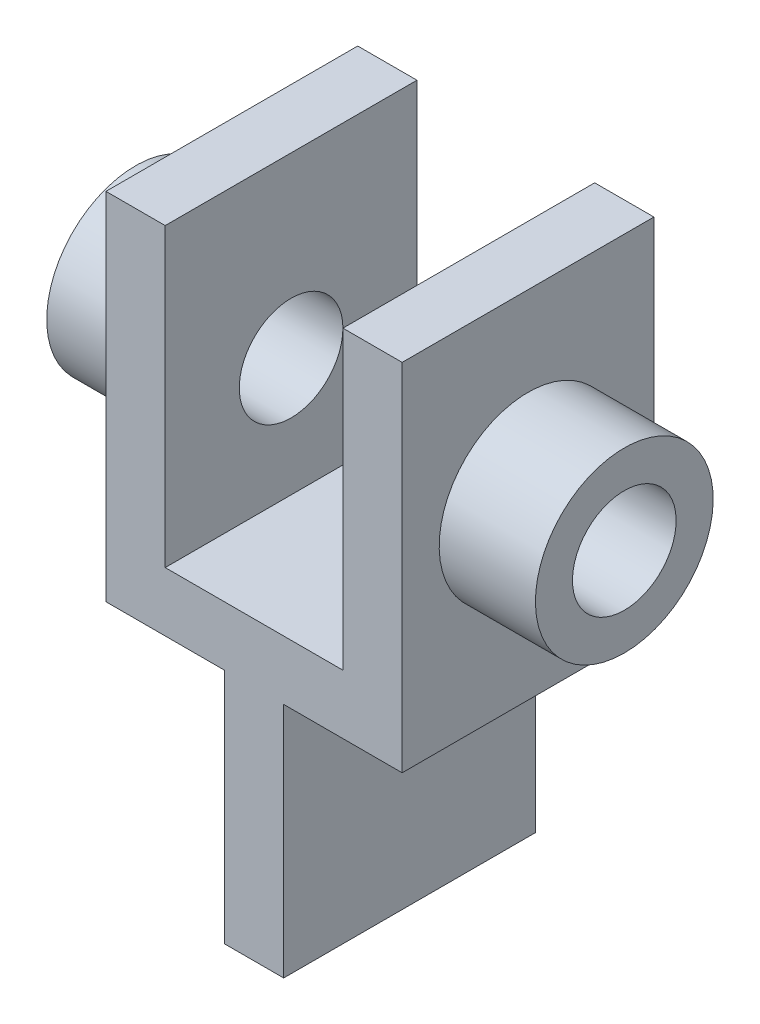
ISO-10303-21;
HEADER;
FILE_DESCRIPTION(('STEP AP214'),'2;1');
FILE_NAME('part.step','',(''),(''),'','','');
FILE_SCHEMA(('AUTOMOTIVE_DESIGN { 1 0 10303 214 1 1 1 1 }'));
ENDSEC;
DATA;
#1=APPLICATION_CONTEXT('core data for automotive mechanical design processes');
#2=APPLICATION_PROTOCOL_DEFINITION('international standard','automotive_design',2000,#1);
#3=PRODUCT_CONTEXT('',#1,'mechanical');
#4=PRODUCT('Part','Part','',(#3));
#5=PRODUCT_RELATED_PRODUCT_CATEGORY('part','',(#4));
#6=PRODUCT_DEFINITION_FORMATION('','',#4);
#7=PRODUCT_DEFINITION_CONTEXT('part definition',#1,'design');
#8=PRODUCT_DEFINITION('design','',#6,#7);
#9=PRODUCT_DEFINITION_SHAPE('','',#8);
#10=(LENGTH_UNIT() NAMED_UNIT(*) SI_UNIT(.MILLI.,.METRE.));
#11=(NAMED_UNIT(*) PLANE_ANGLE_UNIT() SI_UNIT($,.RADIAN.));
#12=(NAMED_UNIT(*) SI_UNIT($,.STERADIAN.) SOLID_ANGLE_UNIT());
#13=UNCERTAINTY_MEASURE_WITH_UNIT(LENGTH_MEASURE(1.E-05),#10,'distance_accuracy_value','');
#14=(GEOMETRIC_REPRESENTATION_CONTEXT(3) GLOBAL_UNCERTAINTY_ASSIGNED_CONTEXT((#13)) GLOBAL_UNIT_ASSIGNED_CONTEXT((#10,
#11,#12)) REPRESENTATION_CONTEXT('',''));
#15=CARTESIAN_POINT('',(0.,0.,0.));
#16=DIRECTION('',(0.,0.,1.));
#17=DIRECTION('',(1.,0.,0.));
#18=AXIS2_PLACEMENT_3D('',#15,#16,#17);
#19=CARTESIAN_POINT('',(-2.8719126938541,0.,-34.));
#20=DIRECTION('',(0.,-1.,0.));
#21=DIRECTION('',(0.,0.,-1.));
#22=AXIS2_PLACEMENT_3D('',#19,#20,#21);
#23=PLANE('',#22);
#24=DIRECTION('',(1.,0.,0.));
#25=VECTOR('',#24,1.);
#26=CARTESIAN_POINT('',(-2.8719126938541,0.,0.));
#27=LINE('',#26,#25);
#28=CARTESIAN_POINT('',(-2.8719126938541,0.,0.));
#29=VERTEX_POINT('',#28);
#30=CARTESIAN_POINT('',(5.1280873061459,0.,0.));
#31=VERTEX_POINT('',#30);
#32=EDGE_CURVE('E165',#29,#31,#27,.T.);
#33=ORIENTED_EDGE('',*,*,#32,.F.);
#34=DIRECTION('',(0.,0.,1.));
#35=VECTOR('',#34,1.);
#36=CARTESIAN_POINT('',(-2.8719126938541,0.,-34.));
#37=LINE('',#36,#35);
#38=CARTESIAN_POINT('',(-2.8719126938541,0.,-34.));
#39=VERTEX_POINT('',#38);
#40=EDGE_CURVE('E11',#39,#29,#37,.T.);
#41=ORIENTED_EDGE('',*,*,#40,.F.);
#42=DIRECTION('',(1.,0.,0.));
#43=VECTOR('',#42,1.);
#44=CARTESIAN_POINT('',(-2.8719126938541,0.,-34.));
#45=LINE('',#44,#43);
#46=CARTESIAN_POINT('',(5.1280873061459,0.,-34.));
#47=VERTEX_POINT('',#46);
#48=EDGE_CURVE('E192',#39,#47,#45,.T.);
#49=ORIENTED_EDGE('',*,*,#48,.T.);
#50=DIRECTION('',(0.,0.,1.));
#51=VECTOR('',#50,1.);
#52=CARTESIAN_POINT('',(5.1280873061459,0.,-34.));
#53=LINE('',#52,#51);
#54=EDGE_CURVE('E42',#47,#31,#53,.T.);
#55=ORIENTED_EDGE('',*,*,#54,.T.);
#56=EDGE_LOOP('',(#33,#41,#49,#55));
#57=FACE_BOUND('',#56,.T.);
#58=ADVANCED_FACE('F41',(#57),#23,.T.);
#59=CARTESIAN_POINT('',(-2.8719126938541,0.,-34.));
#60=DIRECTION('',(-1.,0.,0.));
#61=DIRECTION('',(0.,0.,1.));
#62=AXIS2_PLACEMENT_3D('',#59,#60,#61);
#63=PLANE('',#62);
#64=DIRECTION('',(0.,-1.,0.));
#65=VECTOR('',#64,1.);
#66=CARTESIAN_POINT('',(-2.8719126938541,0.,0.));
#67=LINE('',#66,#65);
#68=CARTESIAN_POINT('',(-2.8719126938541,32.,0.));
#69=VERTEX_POINT('',#68);
#70=EDGE_CURVE('E191',#69,#29,#67,.T.);
#71=ORIENTED_EDGE('',*,*,#70,.F.);
#72=DIRECTION('',(0.,0.,1.));
#73=VECTOR('',#72,1.);
#74=CARTESIAN_POINT('',(-2.8719126938541,32.,-34.));
#75=LINE('',#74,#73);
#76=CARTESIAN_POINT('',(-2.8719126938541,32.,-34.));
#77=VERTEX_POINT('',#76);
#78=EDGE_CURVE('E49',#77,#69,#75,.T.);
#79=ORIENTED_EDGE('',*,*,#78,.F.);
#80=DIRECTION('',(0.,-1.,0.));
#81=VECTOR('',#80,1.);
#82=CARTESIAN_POINT('',(-2.8719126938541,0.,-34.));
#83=LINE('',#82,#81);
#84=EDGE_CURVE('E155',#77,#39,#83,.T.);
#85=ORIENTED_EDGE('',*,*,#84,.T.);
#86=ORIENTED_EDGE('',*,*,#40,.T.);
#87=EDGE_LOOP('',(#71,#79,#85,#86));
#88=FACE_BOUND('',#87,.T.);
#89=ADVANCED_FACE('F214',(#88),#63,.T.);
#90=CARTESIAN_POINT('',(-2.8719126938541,32.,-34.));
#91=DIRECTION('',(0.,-1.,0.));
#92=DIRECTION('',(1.,0.,0.));
#93=AXIS2_PLACEMENT_3D('',#90,#91,#92);
#94=PLANE('',#93);
#95=DIRECTION('',(1.,0.,0.));
#96=VECTOR('',#95,1.);
#97=CARTESIAN_POINT('',(-2.8719126938541,32.,0.));
#98=LINE('',#97,#96);
#99=CARTESIAN_POINT('',(-18.8719126938541,32.,0.));
#100=VERTEX_POINT('',#99);
#101=EDGE_CURVE('E139',#100,#69,#98,.T.);
#102=ORIENTED_EDGE('',*,*,#101,.F.);
#103=DIRECTION('',(0.,0.,1.));
#104=VECTOR('',#103,1.);
#105=CARTESIAN_POINT('',(-18.8719126938541,32.,-34.));
#106=LINE('',#105,#104);
#107=CARTESIAN_POINT('',(-18.8719126938541,32.,-34.));
#108=VERTEX_POINT('',#107);
#109=EDGE_CURVE('E134',#108,#100,#106,.T.);
#110=ORIENTED_EDGE('',*,*,#109,.F.);
#111=DIRECTION('',(1.,0.,0.));
#112=VECTOR('',#111,1.);
#113=CARTESIAN_POINT('',(-2.8719126938541,32.,-34.));
#114=LINE('',#113,#112);
#115=EDGE_CURVE('E140',#108,#77,#114,.T.);
#116=ORIENTED_EDGE('',*,*,#115,.T.);
#117=ORIENTED_EDGE('',*,*,#78,.T.);
#118=EDGE_LOOP('',(#102,#110,#116,#117));
#119=FACE_BOUND('',#118,.T.);
#120=ADVANCED_FACE('F138',(#119),#94,.T.);
#121=CARTESIAN_POINT('',(-18.8719126938541,32.,-34.));
#122=DIRECTION('',(-1.,0.,0.));
#123=DIRECTION('',(0.,0.,1.));
#124=AXIS2_PLACEMENT_3D('',#121,#122,#123);
#125=PLANE('',#124);
#126=CARTESIAN_POINT('',(-18.8719126938541,56.,-17.));
#127=DIRECTION('',(-1.,0.,0.));
#128=DIRECTION('',(0.,0.,1.));
#129=AXIS2_PLACEMENT_3D('',#126,#127,#128);
#130=CIRCLE('',#129,12.);
#131=CARTESIAN_POINT('',(-18.8719126938541,56.,-29.));
#132=VERTEX_POINT('',#131);
#133=EDGE_CURVE('E296',#132,#132,#130,.T.);
#134=ORIENTED_EDGE('',*,*,#133,.F.);
#135=EDGE_LOOP('',(#134));
#136=FACE_BOUND('',#135,.T.);
#137=DIRECTION('',(0.,-1.,0.));
#138=VECTOR('',#137,1.);
#139=CARTESIAN_POINT('',(-18.8719126938541,32.,0.));
#140=LINE('',#139,#138);
#141=CARTESIAN_POINT('',(-18.8719126938541,80.,0.));
#142=VERTEX_POINT('',#141);
#143=EDGE_CURVE('E187',#142,#100,#140,.T.);
#144=ORIENTED_EDGE('',*,*,#143,.F.);
#145=DIRECTION('',(0.,0.,1.));
#146=VECTOR('',#145,1.);
#147=CARTESIAN_POINT('',(-18.8719126938541,80.,-34.));
#148=LINE('',#147,#146);
#149=CARTESIAN_POINT('',(-18.8719126938541,80.,-34.));
#150=VERTEX_POINT('',#149);
#151=EDGE_CURVE('E145',#150,#142,#148,.T.);
#152=ORIENTED_EDGE('',*,*,#151,.F.);
#153=DIRECTION('',(0.,-1.,0.));
#154=VECTOR('',#153,1.);
#155=CARTESIAN_POINT('',(-18.8719126938541,32.,-34.));
#156=LINE('',#155,#154);
#157=EDGE_CURVE('E147',#150,#108,#156,.T.);
#158=ORIENTED_EDGE('',*,*,#157,.T.);
#159=ORIENTED_EDGE('',*,*,#109,.T.);
#160=EDGE_LOOP('',(#144,#152,#158,#159));
#161=FACE_BOUND('',#160,.T.);
#162=ADVANCED_FACE('F152',(#136,#161),#125,.T.);
#163=CARTESIAN_POINT('',(-18.8719126938541,80.,-34.));
#164=DIRECTION('',(0.,1.,0.));
#165=DIRECTION('',(0.,0.,1.));
#166=AXIS2_PLACEMENT_3D('',#163,#164,#165);
#167=PLANE('',#166);
#168=DIRECTION('',(-1.,0.,0.));
#169=VECTOR('',#168,1.);
#170=CARTESIAN_POINT('',(-18.8719126938541,80.,0.));
#171=LINE('',#170,#169);
#172=CARTESIAN_POINT('',(-10.8719126938541,80.,0.));
#173=VERTEX_POINT('',#172);
#174=EDGE_CURVE('E190',#173,#142,#171,.T.);
#175=ORIENTED_EDGE('',*,*,#174,.F.);
#176=DIRECTION('',(0.,0.,1.));
#177=VECTOR('',#176,1.);
#178=CARTESIAN_POINT('',(-10.8719126938541,80.,-34.));
#179=LINE('',#178,#177);
#180=CARTESIAN_POINT('',(-10.8719126938541,80.,-34.));
#181=VERTEX_POINT('',#180);
#182=EDGE_CURVE('E200',#181,#173,#179,.T.);
#183=ORIENTED_EDGE('',*,*,#182,.F.);
#184=DIRECTION('',(-1.,0.,0.));
#185=VECTOR('',#184,1.);
#186=CARTESIAN_POINT('',(-18.8719126938541,80.,-34.));
#187=LINE('',#186,#185);
#188=EDGE_CURVE('E154',#181,#150,#187,.T.);
#189=ORIENTED_EDGE('',*,*,#188,.T.);
#190=ORIENTED_EDGE('',*,*,#151,.T.);
#191=EDGE_LOOP('',(#175,#183,#189,#190));
#192=FACE_BOUND('',#191,.T.);
#193=ADVANCED_FACE('F226',(#192),#167,.T.);
#194=CARTESIAN_POINT('',(-10.8719126938541,80.,-34.));
#195=DIRECTION('',(1.,0.,0.));
#196=DIRECTION('',(0.,1.,0.));
#197=AXIS2_PLACEMENT_3D('',#194,#195,#196);
#198=PLANE('',#197);
#199=CARTESIAN_POINT('',(-10.8719126938541,56.,-17.));
#200=DIRECTION('',(1.,0.,0.));
#201=DIRECTION('',(0.,1.,0.));
#202=AXIS2_PLACEMENT_3D('',#199,#200,#201);
#203=CIRCLE('',#202,7.);
#204=CARTESIAN_POINT('',(-10.8719126938541,56.,-24.));
#205=VERTEX_POINT('',#204);
#206=EDGE_CURVE('E293',#205,#205,#203,.T.);
#207=ORIENTED_EDGE('',*,*,#206,.F.);
#208=EDGE_LOOP('',(#207));
#209=FACE_BOUND('',#208,.T.);
#210=DIRECTION('',(0.,1.,0.));
#211=VECTOR('',#210,1.);
#212=CARTESIAN_POINT('',(-10.8719126938541,80.,0.));
#213=LINE('',#212,#211);
#214=CARTESIAN_POINT('',(-10.8719126938541,40.,0.));
#215=VERTEX_POINT('',#214);
#216=EDGE_CURVE('E184',#215,#173,#213,.T.);
#217=ORIENTED_EDGE('',*,*,#216,.F.);
#218=DIRECTION('',(0.,0.,1.));
#219=VECTOR('',#218,1.);
#220=CARTESIAN_POINT('',(-10.8719126938541,40.,-34.));
#221=LINE('',#220,#219);
#222=CARTESIAN_POINT('',(-10.8719126938541,40.,-34.));
#223=VERTEX_POINT('',#222);
#224=EDGE_CURVE('E203',#223,#215,#221,.T.);
#225=ORIENTED_EDGE('',*,*,#224,.F.);
#226=DIRECTION('',(0.,1.,0.));
#227=VECTOR('',#226,1.);
#228=CARTESIAN_POINT('',(-10.8719126938541,80.,-34.));
#229=LINE('',#228,#227);
#230=EDGE_CURVE('E160',#223,#181,#229,.T.);
#231=ORIENTED_EDGE('',*,*,#230,.T.);
#232=ORIENTED_EDGE('',*,*,#182,.T.);
#233=EDGE_LOOP('',(#217,#225,#231,#232));
#234=FACE_BOUND('',#233,.T.);
#235=ADVANCED_FACE('F235',(#209,#234),#198,.T.);
#236=CARTESIAN_POINT('',(-10.8719126938541,40.,-34.));
#237=DIRECTION('',(0.,1.,0.));
#238=DIRECTION('',(-1.,0.,0.));
#239=AXIS2_PLACEMENT_3D('',#236,#237,#238);
#240=PLANE('',#239);
#241=DIRECTION('',(-1.,0.,0.));
#242=VECTOR('',#241,1.);
#243=CARTESIAN_POINT('',(-10.8719126938541,40.,0.));
#244=LINE('',#243,#242);
#245=CARTESIAN_POINT('',(13.1280873061459,40.,0.));
#246=VERTEX_POINT('',#245);
#247=EDGE_CURVE('E182',#246,#215,#244,.T.);
#248=ORIENTED_EDGE('',*,*,#247,.F.);
#249=DIRECTION('',(0.,0.,1.));
#250=VECTOR('',#249,1.);
#251=CARTESIAN_POINT('',(13.1280873061459,40.,-34.));
#252=LINE('',#251,#250);
#253=CARTESIAN_POINT('',(13.1280873061459,40.,-34.));
#254=VERTEX_POINT('',#253);
#255=EDGE_CURVE('E201',#254,#246,#252,.T.);
#256=ORIENTED_EDGE('',*,*,#255,.F.);
#257=DIRECTION('',(-1.,0.,0.));
#258=VECTOR('',#257,1.);
#259=CARTESIAN_POINT('',(-10.8719126938541,40.,-34.));
#260=LINE('',#259,#258);
#261=EDGE_CURVE('E332',#254,#223,#260,.T.);
#262=ORIENTED_EDGE('',*,*,#261,.T.);
#263=ORIENTED_EDGE('',*,*,#224,.T.);
#264=EDGE_LOOP('',(#248,#256,#262,#263));
#265=FACE_BOUND('',#264,.T.);
#266=ADVANCED_FACE('F237',(#265),#240,.T.);
#267=CARTESIAN_POINT('',(13.1280873061459,40.,-34.));
#268=DIRECTION('',(-1.,0.,0.));
#269=DIRECTION('',(0.,0.,1.));
#270=AXIS2_PLACEMENT_3D('',#267,#268,#269);
#271=PLANE('',#270);
#272=CARTESIAN_POINT('',(13.1280873061459,56.,-17.));
#273=DIRECTION('',(-1.,0.,0.));
#274=DIRECTION('',(0.,0.,1.));
#275=AXIS2_PLACEMENT_3D('',#272,#273,#274);
#276=CIRCLE('',#275,7.);
#277=CARTESIAN_POINT('',(13.1280873061459,49.,-17.));
#278=VERTEX_POINT('',#277);
#279=EDGE_CURVE('E298',#278,#278,#276,.T.);
#280=ORIENTED_EDGE('',*,*,#279,.F.);
#281=EDGE_LOOP('',(#280));
#282=FACE_BOUND('',#281,.T.);
#283=DIRECTION('',(0.,-1.,0.));
#284=VECTOR('',#283,1.);
#285=CARTESIAN_POINT('',(13.1280873061459,40.,0.));
#286=LINE('',#285,#284);
#287=CARTESIAN_POINT('',(13.1280873061459,80.,0.));
#288=VERTEX_POINT('',#287);
#289=EDGE_CURVE('E176',#288,#246,#286,.T.);
#290=ORIENTED_EDGE('',*,*,#289,.F.);
#291=DIRECTION('',(0.,0.,1.));
#292=VECTOR('',#291,1.);
#293=CARTESIAN_POINT('',(13.1280873061459,80.,-34.));
#294=LINE('',#293,#292);
#295=CARTESIAN_POINT('',(13.1280873061459,80.,-34.));
#296=VERTEX_POINT('',#295);
#297=EDGE_CURVE('E202',#296,#288,#294,.T.);
#298=ORIENTED_EDGE('',*,*,#297,.F.);
#299=DIRECTION('',(0.,-1.,0.));
#300=VECTOR('',#299,1.);
#301=CARTESIAN_POINT('',(13.1280873061459,40.,-34.));
#302=LINE('',#301,#300);
#303=EDGE_CURVE('E327',#296,#254,#302,.T.);
#304=ORIENTED_EDGE('',*,*,#303,.T.);
#305=ORIENTED_EDGE('',*,*,#255,.T.);
#306=EDGE_LOOP('',(#290,#298,#304,#305));
#307=FACE_BOUND('',#306,.T.);
#308=ADVANCED_FACE('F238',(#282,#307),#271,.T.);
#309=CARTESIAN_POINT('',(13.1280873061459,80.,-34.));
#310=DIRECTION('',(0.,1.,0.));
#311=DIRECTION('',(0.,0.,1.));
#312=AXIS2_PLACEMENT_3D('',#309,#310,#311);
#313=PLANE('',#312);
#314=DIRECTION('',(-1.,0.,0.));
#315=VECTOR('',#314,1.);
#316=CARTESIAN_POINT('',(13.1280873061459,80.,0.));
#317=LINE('',#316,#315);
#318=CARTESIAN_POINT('',(21.1280873061459,80.,0.));
#319=VERTEX_POINT('',#318);
#320=EDGE_CURVE('E172',#319,#288,#317,.T.);
#321=ORIENTED_EDGE('',*,*,#320,.F.);
#322=DIRECTION('',(0.,0.,1.));
#323=VECTOR('',#322,1.);
#324=CARTESIAN_POINT('',(21.1280873061459,80.,-34.));
#325=LINE('',#324,#323);
#326=CARTESIAN_POINT('',(21.1280873061459,80.,-34.));
#327=VERTEX_POINT('',#326);
#328=EDGE_CURVE('E210',#327,#319,#325,.T.);
#329=ORIENTED_EDGE('',*,*,#328,.F.);
#330=DIRECTION('',(-1.,0.,0.));
#331=VECTOR('',#330,1.);
#332=CARTESIAN_POINT('',(13.1280873061459,80.,-34.));
#333=LINE('',#332,#331);
#334=EDGE_CURVE('E324',#327,#296,#333,.T.);
#335=ORIENTED_EDGE('',*,*,#334,.T.);
#336=ORIENTED_EDGE('',*,*,#297,.T.);
#337=EDGE_LOOP('',(#321,#329,#335,#336));
#338=FACE_BOUND('',#337,.T.);
#339=ADVANCED_FACE('F244',(#338),#313,.T.);
#340=CARTESIAN_POINT('',(21.1280873061459,80.,-34.));
#341=DIRECTION('',(1.,0.,0.));
#342=DIRECTION('',(0.,1.,0.));
#343=AXIS2_PLACEMENT_3D('',#340,#341,#342);
#344=PLANE('',#343);
#345=CARTESIAN_POINT('',(21.1280873061459,56.,-17.));
#346=DIRECTION('',(1.,0.,0.));
#347=DIRECTION('',(0.,1.,0.));
#348=AXIS2_PLACEMENT_3D('',#345,#346,#347);
#349=CIRCLE('',#348,12.);
#350=CARTESIAN_POINT('',(21.1280873061459,44.,-17.));
#351=VERTEX_POINT('',#350);
#352=EDGE_CURVE('E313',#351,#351,#349,.T.);
#353=ORIENTED_EDGE('',*,*,#352,.F.);
#354=EDGE_LOOP('',(#353));
#355=FACE_BOUND('',#354,.T.);
#356=DIRECTION('',(0.,1.,0.));
#357=VECTOR('',#356,1.);
#358=CARTESIAN_POINT('',(21.1280873061459,80.,0.));
#359=LINE('',#358,#357);
#360=CARTESIAN_POINT('',(21.1280873061459,32.,0.));
#361=VERTEX_POINT('',#360);
#362=EDGE_CURVE('E175',#361,#319,#359,.T.);
#363=ORIENTED_EDGE('',*,*,#362,.F.);
#364=DIRECTION('',(0.,0.,1.));
#365=VECTOR('',#364,1.);
#366=CARTESIAN_POINT('',(21.1280873061459,32.,-34.));
#367=LINE('',#366,#365);
#368=CARTESIAN_POINT('',(21.1280873061459,32.,-34.));
#369=VERTEX_POINT('',#368);
#370=EDGE_CURVE('E207',#369,#361,#367,.T.);
#371=ORIENTED_EDGE('',*,*,#370,.F.);
#372=DIRECTION('',(0.,1.,0.));
#373=VECTOR('',#372,1.);
#374=CARTESIAN_POINT('',(21.1280873061459,80.,-34.));
#375=LINE('',#374,#373);
#376=EDGE_CURVE('E325',#369,#327,#375,.T.);
#377=ORIENTED_EDGE('',*,*,#376,.T.);
#378=ORIENTED_EDGE('',*,*,#328,.T.);
#379=EDGE_LOOP('',(#363,#371,#377,#378));
#380=FACE_BOUND('',#379,.T.);
#381=ADVANCED_FACE('F246',(#355,#380),#344,.T.);
#382=CARTESIAN_POINT('',(21.1280873061459,32.,-34.));
#383=DIRECTION('',(0.,-1.,0.));
#384=DIRECTION('',(1.,0.,0.));
#385=AXIS2_PLACEMENT_3D('',#382,#383,#384);
#386=PLANE('',#385);
#387=DIRECTION('',(1.,0.,0.));
#388=VECTOR('',#387,1.);
#389=CARTESIAN_POINT('',(21.1280873061459,32.,0.));
#390=LINE('',#389,#388);
#391=CARTESIAN_POINT('',(5.1280873061459,32.,0.));
#392=VERTEX_POINT('',#391);
#393=EDGE_CURVE('E166',#392,#361,#390,.T.);
#394=ORIENTED_EDGE('',*,*,#393,.F.);
#395=DIRECTION('',(0.,0.,1.));
#396=VECTOR('',#395,1.);
#397=CARTESIAN_POINT('',(5.1280873061459,32.,-34.));
#398=LINE('',#397,#396);
#399=CARTESIAN_POINT('',(5.1280873061459,32.,-34.));
#400=VERTEX_POINT('',#399);
#401=EDGE_CURVE('E209',#400,#392,#398,.T.);
#402=ORIENTED_EDGE('',*,*,#401,.F.);
#403=DIRECTION('',(1.,0.,0.));
#404=VECTOR('',#403,1.);
#405=CARTESIAN_POINT('',(21.1280873061459,32.,-34.));
#406=LINE('',#405,#404);
#407=EDGE_CURVE('E317',#400,#369,#406,.T.);
#408=ORIENTED_EDGE('',*,*,#407,.T.);
#409=ORIENTED_EDGE('',*,*,#370,.T.);
#410=EDGE_LOOP('',(#394,#402,#408,#409));
#411=FACE_BOUND('',#410,.T.);
#412=ADVANCED_FACE('F252',(#411),#386,.T.);
#413=CARTESIAN_POINT('',(5.1280873061459,32.,-34.));
#414=DIRECTION('',(1.,0.,0.));
#415=DIRECTION('',(0.,0.,-1.));
#416=AXIS2_PLACEMENT_3D('',#413,#414,#415);
#417=PLANE('',#416);
#418=DIRECTION('',(0.,1.,0.));
#419=VECTOR('',#418,1.);
#420=CARTESIAN_POINT('',(5.1280873061459,32.,0.));
#421=LINE('',#420,#419);
#422=EDGE_CURVE('E164',#31,#392,#421,.T.);
#423=ORIENTED_EDGE('',*,*,#422,.F.);
#424=ORIENTED_EDGE('',*,*,#54,.F.);
#425=DIRECTION('',(0.,1.,0.));
#426=VECTOR('',#425,1.);
#427=CARTESIAN_POINT('',(5.1280873061459,32.,-34.));
#428=LINE('',#427,#426);
#429=EDGE_CURVE('E320',#47,#400,#428,.T.);
#430=ORIENTED_EDGE('',*,*,#429,.T.);
#431=ORIENTED_EDGE('',*,*,#401,.T.);
#432=EDGE_LOOP('',(#423,#424,#430,#431));
#433=FACE_BOUND('',#432,.T.);
#434=ADVANCED_FACE('F215',(#433),#417,.T.);
#435=CARTESIAN_POINT('',(0.,0.,-34.));
#436=DIRECTION('',(0.,0.,-1.));
#437=DIRECTION('',(-1.,0.,0.));
#438=AXIS2_PLACEMENT_3D('',#435,#436,#437);
#439=PLANE('',#438);
#440=ORIENTED_EDGE('',*,*,#48,.F.);
#441=ORIENTED_EDGE('',*,*,#84,.F.);
#442=ORIENTED_EDGE('',*,*,#115,.F.);
#443=ORIENTED_EDGE('',*,*,#157,.F.);
#444=ORIENTED_EDGE('',*,*,#188,.F.);
#445=ORIENTED_EDGE('',*,*,#230,.F.);
#446=ORIENTED_EDGE('',*,*,#261,.F.);
#447=ORIENTED_EDGE('',*,*,#303,.F.);
#448=ORIENTED_EDGE('',*,*,#334,.F.);
#449=ORIENTED_EDGE('',*,*,#376,.F.);
#450=ORIENTED_EDGE('',*,*,#407,.F.);
#451=ORIENTED_EDGE('',*,*,#429,.F.);
#452=EDGE_LOOP('',(#440,#441,#442,#443,#444,#445,#446,#447,#448,#449,#450,#451));
#453=FACE_BOUND('',#452,.T.);
#454=ADVANCED_FACE('F146',(#453),#439,.T.);
#455=CARTESIAN_POINT('',(0.,0.,0.));
#456=DIRECTION('',(0.,0.,-1.));
#457=DIRECTION('',(-1.,0.,0.));
#458=AXIS2_PLACEMENT_3D('',#455,#456,#457);
#459=PLANE('',#458);
#460=ORIENTED_EDGE('',*,*,#32,.T.);
#461=ORIENTED_EDGE('',*,*,#422,.T.);
#462=ORIENTED_EDGE('',*,*,#393,.T.);
#463=ORIENTED_EDGE('',*,*,#362,.T.);
#464=ORIENTED_EDGE('',*,*,#320,.T.);
#465=ORIENTED_EDGE('',*,*,#289,.T.);
#466=ORIENTED_EDGE('',*,*,#247,.T.);
#467=ORIENTED_EDGE('',*,*,#216,.T.);
#468=ORIENTED_EDGE('',*,*,#174,.T.);
#469=ORIENTED_EDGE('',*,*,#143,.T.);
#470=ORIENTED_EDGE('',*,*,#101,.T.);
#471=ORIENTED_EDGE('',*,*,#70,.T.);
#472=EDGE_LOOP('',(#460,#461,#462,#463,#464,#465,#466,#467,#468,#469,#470,#471));
#473=FACE_BOUND('',#472,.T.);
#474=ADVANCED_FACE('F212',(#473),#459,.F.);
#475=CARTESIAN_POINT('',(34.1280873061459,56.,-17.));
#476=DIRECTION('',(1.,0.,0.));
#477=DIRECTION('',(0.,1.,0.));
#478=AXIS2_PLACEMENT_3D('',#475,#476,#477);
#479=PLANE('',#478);
#480=CARTESIAN_POINT('',(34.1280873061459,56.,-17.));
#481=DIRECTION('',(1.,0.,0.));
#482=DIRECTION('',(0.,1.,0.));
#483=AXIS2_PLACEMENT_3D('',#480,#481,#482);
#484=CIRCLE('',#483,12.);
#485=CARTESIAN_POINT('',(34.1280873061459,44.,-17.));
#486=VERTEX_POINT('',#485);
#487=EDGE_CURVE('E167',#486,#486,#484,.T.);
#488=ORIENTED_EDGE('',*,*,#487,.T.);
#489=EDGE_LOOP('',(#488));
#490=FACE_BOUND('',#489,.T.);
#491=CARTESIAN_POINT('',(34.1280873061459,56.,-17.));
#492=DIRECTION('',(1.,0.,0.));
#493=DIRECTION('',(0.,1.,0.));
#494=AXIS2_PLACEMENT_3D('',#491,#492,#493);
#495=CIRCLE('',#494,7.);
#496=CARTESIAN_POINT('',(34.1280873061459,49.,-17.));
#497=VERTEX_POINT('',#496);
#498=EDGE_CURVE('E308',#497,#497,#495,.T.);
#499=ORIENTED_EDGE('',*,*,#498,.F.);
#500=EDGE_LOOP('',(#499));
#501=FACE_BOUND('',#500,.T.);
#502=ADVANCED_FACE('F263',(#490,#501),#479,.T.);
#503=CARTESIAN_POINT('',(34.1280873061459,56.,-17.));
#504=DIRECTION('',(-1.,0.,0.));
#505=DIRECTION('',(0.,-1.,0.));
#506=AXIS2_PLACEMENT_3D('',#503,#504,#505);
#507=CYLINDRICAL_SURFACE('',#506,12.);
#508=CARTESIAN_POINT('',(34.1280873061459,44.,-17.));
#509=CARTESIAN_POINT('',(33.9926706394792,44.,-17.));
#510=CARTESIAN_POINT('',(33.8572539728126,44.,-17.));
#511=CARTESIAN_POINT('',(33.5864206394792,44.,-17.));
#512=CARTESIAN_POINT('',(33.4510039728126,44.,-17.));
#513=CARTESIAN_POINT('',(33.1801706394793,44.,-17.));
#514=CARTESIAN_POINT('',(33.0447539728126,44.,-17.));
#515=CARTESIAN_POINT('',(32.7739206394792,44.,-17.));
#516=CARTESIAN_POINT('',(32.6385039728126,44.,-17.));
#517=CARTESIAN_POINT('',(32.3676706394793,44.,-17.));
#518=CARTESIAN_POINT('',(32.2322539728126,44.,-17.));
#519=CARTESIAN_POINT('',(31.9614206394792,44.,-17.));
#520=CARTESIAN_POINT('',(31.8260039728126,44.,-17.));
#521=CARTESIAN_POINT('',(31.5551706394792,44.,-17.));
#522=CARTESIAN_POINT('',(31.4197539728126,44.,-17.));
#523=CARTESIAN_POINT('',(31.1489206394792,44.,-17.));
#524=CARTESIAN_POINT('',(31.0135039728126,44.,-17.));
#525=CARTESIAN_POINT('',(30.7426706394792,44.,-17.));
#526=CARTESIAN_POINT('',(30.6072539728126,44.,-17.));
#527=CARTESIAN_POINT('',(30.3364206394792,44.,-17.));
#528=CARTESIAN_POINT('',(30.2010039728126,44.,-17.));
#529=CARTESIAN_POINT('',(29.9301706394792,44.,-17.));
#530=CARTESIAN_POINT('',(29.7947539728126,44.,-17.));
#531=CARTESIAN_POINT('',(29.5239206394792,44.,-17.));
#532=CARTESIAN_POINT('',(29.3885039728126,44.,-17.));
#533=CARTESIAN_POINT('',(29.1176706394792,44.,-17.));
#534=CARTESIAN_POINT('',(28.9822539728126,44.,-17.));
#535=CARTESIAN_POINT('',(28.7114206394792,44.,-17.));
#536=CARTESIAN_POINT('',(28.5760039728126,44.,-17.));
#537=CARTESIAN_POINT('',(28.3051706394792,44.,-17.));
#538=CARTESIAN_POINT('',(28.1697539728126,44.,-17.));
#539=CARTESIAN_POINT('',(27.8989206394792,44.,-17.));
#540=CARTESIAN_POINT('',(27.7635039728126,44.,-17.));
#541=CARTESIAN_POINT('',(27.4926706394792,44.,-17.));
#542=CARTESIAN_POINT('',(27.3572539728126,44.,-17.));
#543=CARTESIAN_POINT('',(27.0864206394792,44.,-17.));
#544=CARTESIAN_POINT('',(26.9510039728126,44.,-17.));
#545=CARTESIAN_POINT('',(26.6801706394792,44.,-17.));
#546=CARTESIAN_POINT('',(26.5447539728126,44.,-17.));
#547=CARTESIAN_POINT('',(26.2739206394792,44.,-17.));
#548=CARTESIAN_POINT('',(26.1385039728126,44.,-17.));
#549=CARTESIAN_POINT('',(25.8676706394792,44.,-17.));
#550=CARTESIAN_POINT('',(25.7322539728126,44.,-17.));
#551=CARTESIAN_POINT('',(25.4614206394792,44.,-17.));
#552=CARTESIAN_POINT('',(25.3260039728126,44.,-17.));
#553=CARTESIAN_POINT('',(25.0551706394792,44.,-17.));
#554=CARTESIAN_POINT('',(24.9197539728126,44.,-17.));
#555=CARTESIAN_POINT('',(24.6489206394792,44.,-17.));
#556=CARTESIAN_POINT('',(24.5135039728126,44.,-17.));
#557=CARTESIAN_POINT('',(24.2426706394792,44.,-17.));
#558=CARTESIAN_POINT('',(24.1072539728126,44.,-17.));
#559=CARTESIAN_POINT('',(23.8364206394792,44.,-17.));
#560=CARTESIAN_POINT('',(23.7010039728126,44.,-17.));
#561=CARTESIAN_POINT('',(23.4301706394792,44.,-17.));
#562=CARTESIAN_POINT('',(23.2947539728126,44.,-17.));
#563=CARTESIAN_POINT('',(23.0239206394792,44.,-17.));
#564=CARTESIAN_POINT('',(22.8885039728126,44.,-17.));
#565=CARTESIAN_POINT('',(22.6176706394792,44.,-17.));
#566=CARTESIAN_POINT('',(22.4822539728126,44.,-17.));
#567=CARTESIAN_POINT('',(22.2114206394792,44.,-17.));
#568=CARTESIAN_POINT('',(22.0760039728126,44.,-17.));
#569=CARTESIAN_POINT('',(21.8051706394792,44.,-17.));
#570=CARTESIAN_POINT('',(21.6697539728126,44.,-17.));
#571=CARTESIAN_POINT('',(21.3989206394792,44.,-17.));
#572=CARTESIAN_POINT('',(21.2635039728126,44.,-17.));
#573=CARTESIAN_POINT('',(21.1280873061459,44.,-17.));
#574=B_SPLINE_CURVE_WITH_KNOTS('',3,(#508,#509,#510,#511,#512,#513,#514,#515,#516,#517,#518,
#519,#520,#521,#522,#523,#524,#525,#526,#527,#528,#529,#530,#531,#532,#533,#534,#535,#536,#537,
#538,#539,#540,#541,#542,#543,#544,#545,#546,#547,#548,#549,#550,#551,#552,#553,#554,#555,#556,
#557,#558,#559,#560,#561,#562,#563,#564,#565,#566,#567,#568,#569,#570,#571,#572,#573),
.UNSPECIFIED.,.F.,.F.,(4,2,2,2,2,2,2,2,2,2,2,2,2,2,2,2,2,2,2,2,2,2,2,2,2,2,2,2,2,2,2,2,4),(0.,
0.406249999999997,0.812499999999994,1.21875,1.62499999999999,2.03125,2.4375,2.84375,3.25,
3.65625,4.0625,4.46875,4.875,5.28125,5.6875,6.09375,6.5,6.90625,7.3125,7.71875,8.125,8.53125,
8.9375,9.34375,9.75,10.15625,10.5625,10.96875,11.375,11.78125,12.1875,12.59375,13.),.UNSPECIFIED.);
#575=EDGE_CURVE('BSEAM264',#486,#351,#574,.T.);
#576=ORIENTED_EDGE('',*,*,#487,.F.);
#577=ORIENTED_EDGE('',*,*,#352,.T.);
#578=ORIENTED_EDGE('',*,*,#575,.T.);
#579=ORIENTED_EDGE('',*,*,#575,.F.);
#580=EDGE_LOOP('',(#576,#578,#577,#579));
#581=FACE_BOUND('',#580,.T.);
#582=ADVANCED_FACE('F264',(#581),#507,.T.);
#583=CARTESIAN_POINT('',(34.1280873061459,56.,-17.));
#584=DIRECTION('',(-1.,0.,0.));
#585=DIRECTION('',(0.,-1.,0.));
#586=AXIS2_PLACEMENT_3D('',#583,#584,#585);
#587=CYLINDRICAL_SURFACE('',#586,7.);
#588=CARTESIAN_POINT('',(34.1280873061459,49.,-17.));
#589=CARTESIAN_POINT('',(33.9093373061459,49.,-17.));
#590=CARTESIAN_POINT('',(33.6905873061459,49.,-17.));
#591=CARTESIAN_POINT('',(33.2530873061459,49.,-17.));
#592=CARTESIAN_POINT('',(33.0343373061459,49.,-17.));
#593=CARTESIAN_POINT('',(32.5968373061459,49.,-17.));
#594=CARTESIAN_POINT('',(32.3780873061459,49.,-17.));
#595=CARTESIAN_POINT('',(31.9405873061459,49.,-17.));
#596=CARTESIAN_POINT('',(31.7218373061459,49.,-17.));
#597=CARTESIAN_POINT('',(31.2843373061459,49.,-17.));
#598=CARTESIAN_POINT('',(31.0655873061459,49.,-17.));
#599=CARTESIAN_POINT('',(30.6280873061459,49.,-17.));
#600=CARTESIAN_POINT('',(30.4093373061459,49.,-17.));
#601=CARTESIAN_POINT('',(29.9718373061459,49.,-17.));
#602=CARTESIAN_POINT('',(29.7530873061459,49.,-17.));
#603=CARTESIAN_POINT('',(29.3155873061459,49.,-17.));
#604=CARTESIAN_POINT('',(29.0968373061459,49.,-17.));
#605=CARTESIAN_POINT('',(28.6593373061459,49.,-17.));
#606=CARTESIAN_POINT('',(28.4405873061459,49.,-17.));
#607=CARTESIAN_POINT('',(28.0030873061459,49.,-17.));
#608=CARTESIAN_POINT('',(27.7843373061459,49.,-17.));
#609=CARTESIAN_POINT('',(27.3468373061459,49.,-17.));
#610=CARTESIAN_POINT('',(27.1280873061459,49.,-17.));
#611=CARTESIAN_POINT('',(26.6905873061459,49.,-17.));
#612=CARTESIAN_POINT('',(26.4718373061459,49.,-17.));
#613=CARTESIAN_POINT('',(26.0343373061459,49.,-17.));
#614=CARTESIAN_POINT('',(25.8155873061459,49.,-17.));
#615=CARTESIAN_POINT('',(25.3780873061459,49.,-17.));
#616=CARTESIAN_POINT('',(25.1593373061459,49.,-17.));
#617=CARTESIAN_POINT('',(24.7218373061459,49.,-17.));
#618=CARTESIAN_POINT('',(24.5030873061459,49.,-17.));
#619=CARTESIAN_POINT('',(24.0655873061459,49.,-17.));
#620=CARTESIAN_POINT('',(23.8468373061459,49.,-17.));
#621=CARTESIAN_POINT('',(23.4093373061459,49.,-17.));
#622=CARTESIAN_POINT('',(23.1905873061459,49.,-17.));
#623=CARTESIAN_POINT('',(22.7530873061459,49.,-17.));
#624=CARTESIAN_POINT('',(22.5343373061459,49.,-17.));
#625=CARTESIAN_POINT('',(22.0968373061459,49.,-17.));
#626=CARTESIAN_POINT('',(21.8780873061459,49.,-17.));
#627=CARTESIAN_POINT('',(21.4405873061459,49.,-17.));
#628=CARTESIAN_POINT('',(21.2218373061459,49.,-17.));
#629=CARTESIAN_POINT('',(20.7843373061459,49.,-17.));
#630=CARTESIAN_POINT('',(20.5655873061459,49.,-17.));
#631=CARTESIAN_POINT('',(20.1280873061459,49.,-17.));
#632=CARTESIAN_POINT('',(19.9093373061459,49.,-17.));
#633=CARTESIAN_POINT('',(19.4718373061459,49.,-17.));
#634=CARTESIAN_POINT('',(19.2530873061459,49.,-17.));
#635=CARTESIAN_POINT('',(18.8155873061459,49.,-17.));
#636=CARTESIAN_POINT('',(18.5968373061459,49.,-17.));
#637=CARTESIAN_POINT('',(18.1593373061459,49.,-17.));
#638=CARTESIAN_POINT('',(17.9405873061459,49.,-17.));
#639=CARTESIAN_POINT('',(17.5030873061459,49.,-17.));
#640=CARTESIAN_POINT('',(17.2843373061459,49.,-17.));
#641=CARTESIAN_POINT('',(16.8468373061459,49.,-17.));
#642=CARTESIAN_POINT('',(16.6280873061459,49.,-17.));
#643=CARTESIAN_POINT('',(16.1905873061459,49.,-17.));
#644=CARTESIAN_POINT('',(15.9718373061459,49.,-17.));
#645=CARTESIAN_POINT('',(15.5343373061459,49.,-17.));
#646=CARTESIAN_POINT('',(15.3155873061459,49.,-17.));
#647=CARTESIAN_POINT('',(14.8780873061459,49.,-17.));
#648=CARTESIAN_POINT('',(14.6593373061459,49.,-17.));
#649=CARTESIAN_POINT('',(14.2218373061459,49.,-17.));
#650=CARTESIAN_POINT('',(14.0030873061459,49.,-17.));
#651=CARTESIAN_POINT('',(13.5655873061459,49.,-17.));
#652=CARTESIAN_POINT('',(13.3468373061459,49.,-17.));
#653=CARTESIAN_POINT('',(13.1280873061459,49.,-17.));
#654=B_SPLINE_CURVE_WITH_KNOTS('',3,(#588,#589,#590,#591,#592,#593,#594,#595,#596,#597,#598,
#599,#600,#601,#602,#603,#604,#605,#606,#607,#608,#609,#610,#611,#612,#613,#614,#615,#616,#617,
#618,#619,#620,#621,#622,#623,#624,#625,#626,#627,#628,#629,#630,#631,#632,#633,#634,#635,#636,
#637,#638,#639,#640,#641,#642,#643,#644,#645,#646,#647,#648,#649,#650,#651,#652,#653),
.UNSPECIFIED.,.F.,.F.,(4,2,2,2,2,2,2,2,2,2,2,2,2,2,2,2,2,2,2,2,2,2,2,2,2,2,2,2,2,2,2,2,4),(0.,
0.656250000000004,1.3125,1.96875000000001,2.625,3.28125,3.9375,4.59375,5.25,5.90625000000001,
6.56250000000001,7.21875000000001,7.87500000000001,8.53125,9.18750000000001,9.84375000000001,
10.5,11.15625,11.8125,12.46875,13.125,13.78125,14.4375,15.09375,15.75,16.40625,17.0625,17.71875,
18.375,19.03125,19.6875,20.34375,21.),.UNSPECIFIED.);
#655=EDGE_CURVE('BSEAM268',#497,#278,#654,.T.);
#656=ORIENTED_EDGE('',*,*,#498,.T.);
#657=ORIENTED_EDGE('',*,*,#279,.T.);
#658=ORIENTED_EDGE('',*,*,#655,.T.);
#659=ORIENTED_EDGE('',*,*,#655,.F.);
#660=EDGE_LOOP('',(#656,#658,#657,#659));
#661=FACE_BOUND('',#660,.T.);
#662=ADVANCED_FACE('F268',(#661),#587,.F.);
#663=CARTESIAN_POINT('',(-31.8719126938541,56.,-17.));
#664=DIRECTION('',(-1.,0.,0.));
#665=DIRECTION('',(0.,0.,1.));
#666=AXIS2_PLACEMENT_3D('',#663,#664,#665);
#667=PLANE('',#666);
#668=CARTESIAN_POINT('',(-31.8719126938541,56.,-17.));
#669=DIRECTION('',(-1.,0.,0.));
#670=DIRECTION('',(0.,0.,1.));
#671=AXIS2_PLACEMENT_3D('',#668,#669,#670);
#672=CIRCLE('',#671,12.);
#673=CARTESIAN_POINT('',(-31.8719126938541,56.,-29.));
#674=VERTEX_POINT('',#673);
#675=EDGE_CURVE('E301',#674,#674,#672,.T.);
#676=ORIENTED_EDGE('',*,*,#675,.T.);
#677=EDGE_LOOP('',(#676));
#678=FACE_BOUND('',#677,.T.);
#679=CARTESIAN_POINT('',(-31.8719126938541,56.,-17.));
#680=DIRECTION('',(-1.,0.,0.));
#681=DIRECTION('',(0.,0.,1.));
#682=AXIS2_PLACEMENT_3D('',#679,#680,#681);
#683=CIRCLE('',#682,7.);
#684=CARTESIAN_POINT('',(-31.8719126938541,56.,-24.));
#685=VERTEX_POINT('',#684);
#686=EDGE_CURVE('E295',#685,#685,#683,.T.);
#687=ORIENTED_EDGE('',*,*,#686,.F.);
#688=EDGE_LOOP('',(#687));
#689=FACE_BOUND('',#688,.T.);
#690=ADVANCED_FACE('F274',(#678,#689),#667,.T.);
#691=CARTESIAN_POINT('',(-31.8719126938541,56.,-17.));
#692=DIRECTION('',(1.,0.,0.));
#693=DIRECTION('',(0.,0.,-1.));
#694=AXIS2_PLACEMENT_3D('',#691,#692,#693);
#695=CYLINDRICAL_SURFACE('',#694,12.);
#696=CARTESIAN_POINT('',(-31.8719126938541,56.,-29.));
#697=CARTESIAN_POINT('',(-31.7364960271874,56.,-29.));
#698=CARTESIAN_POINT('',(-31.6010793605208,56.,-29.));
#699=CARTESIAN_POINT('',(-31.3302460271874,56.,-29.));
#700=CARTESIAN_POINT('',(-31.1948293605208,56.,-29.));
#701=CARTESIAN_POINT('',(-30.9239960271874,56.,-29.));
#702=CARTESIAN_POINT('',(-30.7885793605208,56.,-29.));
#703=CARTESIAN_POINT('',(-30.5177460271874,56.,-29.));
#704=CARTESIAN_POINT('',(-30.3823293605208,56.,-29.));
#705=CARTESIAN_POINT('',(-30.1114960271874,56.,-29.));
#706=CARTESIAN_POINT('',(-29.9760793605208,56.,-29.));
#707=CARTESIAN_POINT('',(-29.7052460271874,56.,-29.));
#708=CARTESIAN_POINT('',(-29.5698293605208,56.,-29.));
#709=CARTESIAN_POINT('',(-29.2989960271874,56.,-29.));
#710=CARTESIAN_POINT('',(-29.1635793605208,56.,-29.));
#711=CARTESIAN_POINT('',(-28.8927460271874,56.,-29.));
#712=CARTESIAN_POINT('',(-28.7573293605208,56.,-29.));
#713=CARTESIAN_POINT('',(-28.4864960271874,56.,-29.));
#714=CARTESIAN_POINT('',(-28.3510793605208,56.,-29.));
#715=CARTESIAN_POINT('',(-28.0802460271874,56.,-29.));
#716=CARTESIAN_POINT('',(-27.9448293605208,56.,-29.));
#717=CARTESIAN_POINT('',(-27.6739960271874,56.,-29.));
#718=CARTESIAN_POINT('',(-27.5385793605208,56.,-29.));
#719=CARTESIAN_POINT('',(-27.2677460271874,56.,-29.));
#720=CARTESIAN_POINT('',(-27.1323293605208,56.,-29.));
#721=CARTESIAN_POINT('',(-26.8614960271874,56.,-29.));
#722=CARTESIAN_POINT('',(-26.7260793605208,56.,-29.));
#723=CARTESIAN_POINT('',(-26.4552460271874,56.,-29.));
#724=CARTESIAN_POINT('',(-26.3198293605208,56.,-29.));
#725=CARTESIAN_POINT('',(-26.0489960271874,56.,-29.));
#726=CARTESIAN_POINT('',(-25.9135793605208,56.,-29.));
#727=CARTESIAN_POINT('',(-25.6427460271874,56.,-29.));
#728=CARTESIAN_POINT('',(-25.5073293605208,56.,-29.));
#729=CARTESIAN_POINT('',(-25.2364960271874,56.,-29.));
#730=CARTESIAN_POINT('',(-25.1010793605208,56.,-29.));
#731=CARTESIAN_POINT('',(-24.8302460271874,56.,-29.));
#732=CARTESIAN_POINT('',(-24.6948293605208,56.,-29.));
#733=CARTESIAN_POINT('',(-24.4239960271874,56.,-29.));
#734=CARTESIAN_POINT('',(-24.2885793605208,56.,-29.));
#735=CARTESIAN_POINT('',(-24.0177460271874,56.,-29.));
#736=CARTESIAN_POINT('',(-23.8823293605208,56.,-29.));
#737=CARTESIAN_POINT('',(-23.6114960271874,56.,-29.));
#738=CARTESIAN_POINT('',(-23.4760793605208,56.,-29.));
#739=CARTESIAN_POINT('',(-23.2052460271874,56.,-29.));
#740=CARTESIAN_POINT('',(-23.0698293605208,56.,-29.));
#741=CARTESIAN_POINT('',(-22.7989960271874,56.,-29.));
#742=CARTESIAN_POINT('',(-22.6635793605208,56.,-29.));
#743=CARTESIAN_POINT('',(-22.3927460271874,56.,-29.));
#744=CARTESIAN_POINT('',(-22.2573293605208,56.,-29.));
#745=CARTESIAN_POINT('',(-21.9864960271874,56.,-29.));
#746=CARTESIAN_POINT('',(-21.8510793605208,56.,-29.));
#747=CARTESIAN_POINT('',(-21.5802460271874,56.,-29.));
#748=CARTESIAN_POINT('',(-21.4448293605208,56.,-29.));
#749=CARTESIAN_POINT('',(-21.1739960271874,56.,-29.));
#750=CARTESIAN_POINT('',(-21.0385793605208,56.,-29.));
#751=CARTESIAN_POINT('',(-20.7677460271874,56.,-29.));
#752=CARTESIAN_POINT('',(-20.6323293605208,56.,-29.));
#753=CARTESIAN_POINT('',(-20.3614960271874,56.,-29.));
#754=CARTESIAN_POINT('',(-20.2260793605208,56.,-29.));
#755=CARTESIAN_POINT('',(-19.9552460271874,56.,-29.));
#756=CARTESIAN_POINT('',(-19.8198293605208,56.,-29.));
#757=CARTESIAN_POINT('',(-19.5489960271874,56.,-29.));
#758=CARTESIAN_POINT('',(-19.4135793605208,56.,-29.));
#759=CARTESIAN_POINT('',(-19.1427460271874,56.,-29.));
#760=CARTESIAN_POINT('',(-19.0073293605208,56.,-29.));
#761=CARTESIAN_POINT('',(-18.8719126938541,56.,-29.));
#762=B_SPLINE_CURVE_WITH_KNOTS('',3,(#696,#697,#698,#699,#700,#701,#702,#703,#704,#705,#706,
#707,#708,#709,#710,#711,#712,#713,#714,#715,#716,#717,#718,#719,#720,#721,#722,#723,#724,#725,
#726,#727,#728,#729,#730,#731,#732,#733,#734,#735,#736,#737,#738,#739,#740,#741,#742,#743,#744,
#745,#746,#747,#748,#749,#750,#751,#752,#753,#754,#755,#756,#757,#758,#759,#760,#761),
.UNSPECIFIED.,.F.,.F.,(4,2,2,2,2,2,2,2,2,2,2,2,2,2,2,2,2,2,2,2,2,2,2,2,2,2,2,2,2,2,2,2,4),(0.,
0.406249999999997,0.812499999999997,1.21875,1.625,2.03124999999999,2.4375,2.84375,3.25,3.65625,
4.0625,4.46875,4.875,5.28124999999999,5.6875,6.09374999999999,6.5,6.90625,7.3125,7.71875,
8.12499999999999,8.53125,8.93749999999999,9.34375,9.74999999999999,10.15625,10.5625,10.96875,
11.375,11.78125,12.1875,12.59375,13.),.UNSPECIFIED.);
#763=EDGE_CURVE('BSEAM280',#674,#132,#762,.T.);
#764=ORIENTED_EDGE('',*,*,#675,.F.);
#765=ORIENTED_EDGE('',*,*,#133,.T.);
#766=ORIENTED_EDGE('',*,*,#763,.T.);
#767=ORIENTED_EDGE('',*,*,#763,.F.);
#768=EDGE_LOOP('',(#764,#766,#765,#767));
#769=FACE_BOUND('',#768,.T.);
#770=ADVANCED_FACE('F280',(#769),#695,.T.);
#771=CARTESIAN_POINT('',(-31.8719126938541,56.,-17.));
#772=DIRECTION('',(1.,0.,0.));
#773=DIRECTION('',(0.,0.,-1.));
#774=AXIS2_PLACEMENT_3D('',#771,#772,#773);
#775=CYLINDRICAL_SURFACE('',#774,7.);
#776=CARTESIAN_POINT('',(-31.8719126938541,56.,-24.));
#777=CARTESIAN_POINT('',(-31.6531626938541,56.,-24.));
#778=CARTESIAN_POINT('',(-31.4344126938541,56.,-24.));
#779=CARTESIAN_POINT('',(-30.9969126938541,56.,-24.));
#780=CARTESIAN_POINT('',(-30.7781626938541,56.,-24.));
#781=CARTESIAN_POINT('',(-30.3406626938541,56.,-24.));
#782=CARTESIAN_POINT('',(-30.1219126938541,56.,-24.));
#783=CARTESIAN_POINT('',(-29.6844126938541,56.,-24.));
#784=CARTESIAN_POINT('',(-29.4656626938541,56.,-24.));
#785=CARTESIAN_POINT('',(-29.0281626938541,56.,-24.));
#786=CARTESIAN_POINT('',(-28.8094126938541,56.,-24.));
#787=CARTESIAN_POINT('',(-28.3719126938541,56.,-24.));
#788=CARTESIAN_POINT('',(-28.1531626938541,56.,-24.));
#789=CARTESIAN_POINT('',(-27.7156626938541,56.,-24.));
#790=CARTESIAN_POINT('',(-27.4969126938541,56.,-24.));
#791=CARTESIAN_POINT('',(-27.0594126938541,56.,-24.));
#792=CARTESIAN_POINT('',(-26.8406626938541,56.,-24.));
#793=CARTESIAN_POINT('',(-26.4031626938541,56.,-24.));
#794=CARTESIAN_POINT('',(-26.1844126938541,56.,-24.));
#795=CARTESIAN_POINT('',(-25.7469126938541,56.,-24.));
#796=CARTESIAN_POINT('',(-25.5281626938541,56.,-24.));
#797=CARTESIAN_POINT('',(-25.0906626938541,56.,-24.));
#798=CARTESIAN_POINT('',(-24.8719126938541,56.,-24.));
#799=CARTESIAN_POINT('',(-24.4344126938541,56.,-24.));
#800=CARTESIAN_POINT('',(-24.2156626938541,56.,-24.));
#801=CARTESIAN_POINT('',(-23.7781626938541,56.,-24.));
#802=CARTESIAN_POINT('',(-23.5594126938541,56.,-24.));
#803=CARTESIAN_POINT('',(-23.1219126938541,56.,-24.));
#804=CARTESIAN_POINT('',(-22.9031626938541,56.,-24.));
#805=CARTESIAN_POINT('',(-22.4656626938541,56.,-24.));
#806=CARTESIAN_POINT('',(-22.2469126938541,56.,-24.));
#807=CARTESIAN_POINT('',(-21.8094126938541,56.,-24.));
#808=CARTESIAN_POINT('',(-21.5906626938541,56.,-24.));
#809=CARTESIAN_POINT('',(-21.1531626938541,56.,-24.));
#810=CARTESIAN_POINT('',(-20.9344126938541,56.,-24.));
#811=CARTESIAN_POINT('',(-20.4969126938541,56.,-24.));
#812=CARTESIAN_POINT('',(-20.2781626938541,56.,-24.));
#813=CARTESIAN_POINT('',(-19.8406626938541,56.,-24.));
#814=CARTESIAN_POINT('',(-19.6219126938541,56.,-24.));
#815=CARTESIAN_POINT('',(-19.1844126938541,56.,-24.));
#816=CARTESIAN_POINT('',(-18.9656626938541,56.,-24.));
#817=CARTESIAN_POINT('',(-18.5281626938541,56.,-24.));
#818=CARTESIAN_POINT('',(-18.3094126938541,56.,-24.));
#819=CARTESIAN_POINT('',(-17.8719126938541,56.,-24.));
#820=CARTESIAN_POINT('',(-17.6531626938541,56.,-24.));
#821=CARTESIAN_POINT('',(-17.2156626938541,56.,-24.));
#822=CARTESIAN_POINT('',(-16.9969126938541,56.,-24.));
#823=CARTESIAN_POINT('',(-16.5594126938541,56.,-24.));
#824=CARTESIAN_POINT('',(-16.3406626938541,56.,-24.));
#825=CARTESIAN_POINT('',(-15.9031626938541,56.,-24.));
#826=CARTESIAN_POINT('',(-15.6844126938541,56.,-24.));
#827=CARTESIAN_POINT('',(-15.2469126938541,56.,-24.));
#828=CARTESIAN_POINT('',(-15.0281626938541,56.,-24.));
#829=CARTESIAN_POINT('',(-14.5906626938541,56.,-24.));
#830=CARTESIAN_POINT('',(-14.3719126938541,56.,-24.));
#831=CARTESIAN_POINT('',(-13.9344126938541,56.,-24.));
#832=CARTESIAN_POINT('',(-13.7156626938541,56.,-24.));
#833=CARTESIAN_POINT('',(-13.2781626938541,56.,-24.));
#834=CARTESIAN_POINT('',(-13.0594126938541,56.,-24.));
#835=CARTESIAN_POINT('',(-12.6219126938541,56.,-24.));
#836=CARTESIAN_POINT('',(-12.4031626938541,56.,-24.));
#837=CARTESIAN_POINT('',(-11.9656626938541,56.,-24.));
#838=CARTESIAN_POINT('',(-11.7469126938541,56.,-24.));
#839=CARTESIAN_POINT('',(-11.3094126938541,56.,-24.));
#840=CARTESIAN_POINT('',(-11.0906626938541,56.,-24.));
#841=CARTESIAN_POINT('',(-10.8719126938541,56.,-24.));
#842=B_SPLINE_CURVE_WITH_KNOTS('',3,(#776,#777,#778,#779,#780,#781,#782,#783,#784,#785,#786,
#787,#788,#789,#790,#791,#792,#793,#794,#795,#796,#797,#798,#799,#800,#801,#802,#803,#804,#805,
#806,#807,#808,#809,#810,#811,#812,#813,#814,#815,#816,#817,#818,#819,#820,#821,#822,#823,#824,
#825,#826,#827,#828,#829,#830,#831,#832,#833,#834,#835,#836,#837,#838,#839,#840,#841),
.UNSPECIFIED.,.F.,.F.,(4,2,2,2,2,2,2,2,2,2,2,2,2,2,2,2,2,2,2,2,2,2,2,2,2,2,2,2,2,2,2,2,4),(0.,
0.656250000000004,1.3125,1.96875,2.625,3.28125,3.9375,4.59375,5.25,5.90625,6.5625,7.21875,7.875,
8.53125,9.1875,9.84375,10.5,11.15625,11.8125,12.46875,13.125,13.78125,14.4375,15.09375,15.75,
16.40625,17.0625,17.71875,18.375,19.03125,19.6875,20.34375,21.),.UNSPECIFIED.);
#843=EDGE_CURVE('BSEAM278',#685,#205,#842,.T.);
#844=ORIENTED_EDGE('',*,*,#686,.T.);
#845=ORIENTED_EDGE('',*,*,#206,.T.);
#846=ORIENTED_EDGE('',*,*,#843,.T.);
#847=ORIENTED_EDGE('',*,*,#843,.F.);
#848=EDGE_LOOP('',(#844,#846,#845,#847));
#849=FACE_BOUND('',#848,.T.);
#850=ADVANCED_FACE('F278',(#849),#775,.F.);
#851=CLOSED_SHELL('',(#58,#89,#120,#162,#193,#235,#266,#308,#339,#381,#412,#434,#454,#474,#502,
#582,#662,#690,#770,#850));
#852=MANIFOLD_SOLID_BREP('B2',#851);
#853=ADVANCED_BREP_SHAPE_REPRESENTATION('',(#18,#852),#14);
#854=SHAPE_DEFINITION_REPRESENTATION(#9,#853);
ENDSEC;
END-ISO-10303-21;
